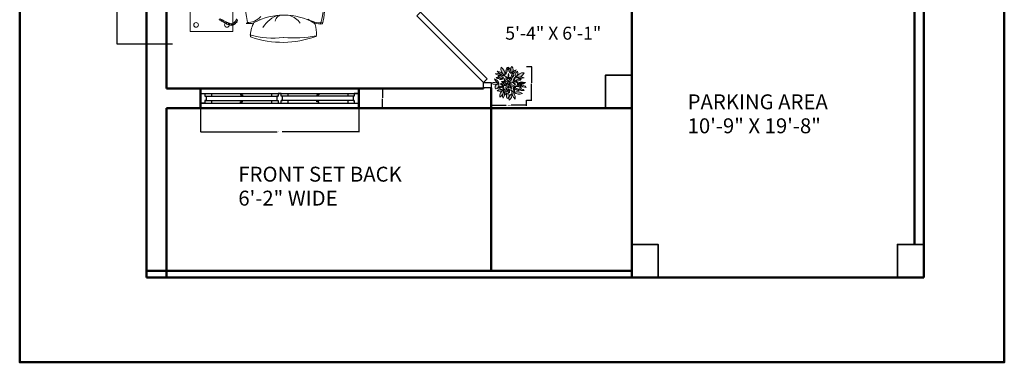
# Model space of a CAD drawing. Units: inches. Extents: x 64 to 1167, y 117 to 939.
# Tile 1 of 56: x 64 to 513, y 117 to 272. Entities that reach past the tile are written whole.
import ezdxf

# ---------------------------------------------------------------- set-up
doc = ezdxf.new("R2010")
doc.units = ezdxf.units.IN
doc.header["$MEASUREMENT"] = 0
for name, color, linetype, lineweight in [('A-ANNO-DIMS', 2, 'Continuous', 18), ('A-ANNO-TEXT', 7, 'Continuous', 25), ('A-ANNO-TTLB', 7, 'Continuous', 50), ('A-COLS', 7, 'Continuous', 35), ('A-DOOR', 4, 'Continuous', 25), ('A-FURN', 8, 'Continuous', 18), ('A-GLAZ', 4, 'Continuous', 25), ('A-WALL', 7, 'Continuous', 50)]:
    doc.layers.add(name, color=color, linetype=linetype, lineweight=lineweight)
doc.styles.get("Standard").update_dxf_attribs({"font": 'arial.ttf'})
doc.dimstyles.get("Standard").update_dxf_attribs({"dimtxt": 0.18, "dimasz": 0.18, "dimexe": 0.18, "dimexo": 0.0625, "dimgap": 0.09, "dimtad": 0, "dimtih": 1, "dimtoh": 1, "dimdec": 4, "dimzin": 0, "dimdsep": 46, "dimtxsty": 'Standard', "dimcen": 0.09, "dimadec": 0, "dimazin": 0, "dimtfac": 1, "dimtdec": 4, "dimtofl": 0, "dimtmove": 0, "dimatfit": 3, "dimfxl": 1, "dimtolj": 1, "dimtzin": 0, "dimarcsym": 0})

# ---------------------------------------------------------------- blocks, each defined once
blk = doc.blocks.new('A$C68901CC0')
for p, q in [((10.95, 26.62), (12.35, 28.01)), ((36.01, 1.56), (10.95, 26.62)), ((12.35, 28.01), (37.4, 2.95)), ((0, 2.95), (0, 0)), ((1.97, 2.95), (0, 2.95)), ((0, 0), (1.97, 0)), ((1.97, 0), (1.97, 2.95)), ((37.4, 2.95), (36.01, 1.56)), ((37.4, 2.95), (37.4, 0)), ((39.37, 2.95), (37.4, 2.95)), ((37.4, 0), (39.37, 0)), ((39.37, 0), (39.37, 2.95))]:
    blk.add_line(p, q)
blk.add_arc((37.4, 2.95), 35.43, 135, 180)
blk = doc.blocks.new("W-6'")
for p, q in [((0, 9), (0, 0)), ((0, 9), (72, 9)), ((72, 9), (72, 0)), ((0, 6.75), (72, 6.75)), ((2, 5.5), (35.25, 5.5)), ((70, 5.5), (36.75, 5.5)), ((0, 2.25), (72, 2.25)), ((0, 0), (72, 0)), ((2, 3.5), (35.25, 3.5)), ((70, 3.5), (36.75, 3.5))]:
    blk.add_line(p, q)
for points in [[(0, 2.25), (0, 6.75), (2, 6.75), (2, 5.5), (2.5, 5.5), (2.5, 3.5), (2, 3.5), (2, 2.25), (0, 2.25)], [(5, 6.75), (5, 5.5)], [(18.125, 6.75), (18.125, 6.125), (19.125, 6.125), (19.125, 5.5)], [(32.25, 6.75), (32.25, 5.5)], [(39.75, 6.75), (39.75, 5.5)], [(53.875, 6.75), (53.875, 6.125), (52.875, 6.125), (52.875, 5.5)], [(67, 6.75), (67, 5.5)], [(72, 2.25), (72, 6.75), (70, 6.75), (70, 5.5), (69.5, 5.5), (69.5, 3.5), (70, 3.5), (70, 2.25), (72, 2.25)], [(5, 3.5), (5, 2.25)], [(18.125, 2.25), (18.125, 2.875), (19.125, 2.875), (19.125, 3.5)], [(32.25, 3.5), (32.25, 2.25)], [(39.75, 3.5), (39.75, 2.25)], [(53.875, 2.25), (53.875, 2.875), (52.875, 2.875), (52.875, 3.5)], [(67, 3.5), (67, 2.25)]]:
    blk.add_lwpolyline(points)
blk.add_lwpolyline([(36.75, 6.75), (35.25, 6.75), (35.25, 5.5), (34.75, 5.5), (34.75, 3.5), (35.25, 3.5), (35.25, 2.25), (36.75, 2.25), (36.75, 3.5), (37.25, 3.5), (37.25, 5.5), (36.75, 5.5)], close=True)
blk = doc.blocks.new('A$C28C76B35')
for p, q in [((66.74, 162.49, -24.36), (86.28, 162.49, -24.36)), ((66.74, 137.72, -24.36), (66.74, 162.49, -24.36)), ((86.28, 162.49, -24.36), (86.28, 137.72, -24.36)), ((64.63, 157.46, -55.71), (64.77, 157.76, -55.71)), ((65, 157.04, -55.71), (64.63, 157.46, -55.71)), ((64.77, 157.76, -55.71), (65.33, 157.7, -55.71)), ((64.85, 158.09, -55.71), (65.11, 158.39, -55.71)), ((65.33, 157.7, -55.71), (64.85, 158.09, -55.71)), ((65.11, 158.39, -55.71), (65.61, 158.17, -55.71)), ((65.63, 157.82, -55.71), (65.16, 156.74, -55.71)), ((65.39, 158.69, -55.71), (65.61, 158.93, -55.71)), ((65.61, 158.17, -55.71), (65.39, 158.69, -55.71)), ((65.61, 158.93, -55.71), (66.11, 158.67, -55.71)), ((66.43, 158.63, -55.71), (65.63, 157.82, -55.71)), ((65.94, 159.21, -55.71), (66.32, 159.36, -55.71)), ((66.11, 158.67, -55.71), (65.94, 159.21, -55.71)), ((66.32, 159.36, -55.71), (66.82, 158.91, -55.71)), ((67.82, 158.89, -55.71), (66.43, 158.63, -55.71)), ((66.79, 159.49, 50.88), (67.17, 159.56, 50.88)), ((66.82, 158.91, -55.71), (66.8, 159.49, -55.71)), ((67.17, 159.56, -55.71), (67.45, 159.08, -55.71)), ((67.45, 159.08, -55.71), (67.62, 159.65, -55.71)), ((67.61, 159.66, 50.88), (68.08, 159.57, 50.88)), ((69.56, 158.28, -55.71), (67.82, 158.89, -55.71)), ((68.08, 159.56, -55.71), (68.08, 159.06, -55.71)), ((68.08, 159.06, -55.71), (68.45, 159.45, -55.71)), ((68.44, 159.45, 50.88), (68.87, 159.32, 50.88)), ((68.88, 159.32, -55.71), (68.86, 158.73, -55.71)), ((68.86, 158.73, -55.71), (69.06, 159.26, -55.71)), ((69.06, 159.26, -55.71), (69.62, 159.1, -55.71)), ((69.62, 159.1, -55.71), (69.56, 158.54, -55.71)), ((69.56, 158.54, -55.71), (70.1, 158.87, -55.71)), ((70.64, 157.69, -55.71), (69.56, 158.28, -55.71)), ((70.1, 158.87, -55.71), (70.4, 158.67, -55.71)), ((70.4, 158.67, -55.71), (70.25, 158.15, -55.71)), ((70.25, 158.15, -55.71), (70.75, 158.43, -55.71)), ((70.79, 157.74, -55.71), (70.64, 157.69, -55.71)), ((70.75, 158.43, -55.71), (71.14, 158.22, -55.71)), ((70.83, 157.61, -55.71), (70.79, 157.74, -55.71)), ((71.59, 157.22, -55.71), (70.83, 157.61, -55.71)), ((71.14, 158.22, -55.71), (70.98, 157.72, -55.71)), ((70.98, 157.72, -55.71), (71.4, 158.06, -55.71)), ((71.4, 158.06, -55.71), (71.81, 157.87, -55.71)), ((71.81, 157.87, -55.71), (71.59, 157.37, -55.71)), ((71.59, 157.37, -55.71), (72.01, 157.76, -55.71)), ((72.59, 156.63, -55.71), (71.59, 157.22, -55.71)), ((72.01, 157.76, -55.71), (72.31, 157.61, -55.71)), ((72.31, 157.61, -55.71), (72.14, 157.07, -55.71)), ((72.14, 157.07, -55.71), (72.68, 157.37, -55.71)), ((72.68, 157.37, -55.71), (72.96, 157.22, -55.71)), ((72.96, 157.22, -55.71), (72.81, 156.74, -55.71))]:
    blk.add_line(p, q)
for centre in [(69.47, 159.47, -27.2), (83.55, 159.47, -27.2)]:
    blk.add_circle(centre, 1.07)
for centre, radius, start, end in [((44.19, 123.6, -100.22), 43.8, 71.1157, 110.2204), ((29.35, 164.01, -100.22), 0.74, 113.3322, 161.3637), ((45.92, 164.21, -100.22), 17.27, 179.879, 196.6328), ((29.34, 164.01, -100.22), 0.74, 114.0758, 156.3315), ((38.67, 116, -100.22), 49.39, 84.253, 101.4358), ((48.54, 128.59, -100.22), 36.87, 73.3816, 97.55), ((47.45, 164.2, -100.22), 11.31, 332.1884, 2.3768), ((58.09, 164.35, -100.22), 0.74, 25.7033, 68.2144), ((90.3, 145.69, -100.22), 65.74, 168.3019, 188.2166), ((77.92, 144.85, -100.22), 52.97, 164.4911, 189.2138), ((26.82, 151.23, -100.22), 7.84, 69.9615, 96.5551), ((26.79, 147.45, -100.22), 11.05, 58.4292, 93.73), ((30.11, 159.24, -100.22), 0.74, 177.437, 237.6208), ((30.11, 159.24, -100.22), 0.74, 178.0201, 240.7828), ((30.13, 158.98, -100.22), 0.74, 184.7243, 243.4779), ((43.65, 183.47, -100.22), 28.49, 240.7828, 298.0488), ((27.78, 151.92, -100.22), 6.89, 46.9453, 51.4779), ((44.46, 165.16, -100.22), 10.65, 217.955, 250.4125), ((44.45, 157.99, -100.22), 3.03, 261.0221, 354.0715), ((42.56, 166.77, -100.22), 12.19, 284.9836, 329.7062), ((60.3, 149.77, -100.22), 8.6, 88.8733, 136.7696), ((59.08, 151.92, -100.22), 6.89, 128.5221, 133.0547), ((56.72, 158.98, -100.22), 0.74, 296.5221, 355.2757), ((59.4, 151.99, -100.22), 6.91, 78.8784, 107.2062), ((-1.21, 144.26, -100.22), 62.88, 353.0352, 12.9689)]:
    blk.add_arc(centre, radius, start, end)
blk = doc.blocks.new('A$C172C5132')
at = {"linetype": 'ByBlock'}
h = blk.add_hatch(color=256, dxfattribs=at)
h.set_gradient(color1=(12, 110, 14), color2=(39, 78, 9), tint=1, name='HEMISPHERICAL')
h.paths.add_polyline_path([(0.0278, 0.1013, 0.287265), (0.0517, 0.0926, 0.287265)])
h.paths.add_polyline_path([(0.0334, 0.0874, 0.245454), (0.05, 0.09, 0.245454)])
h.paths.add_polyline_path([(0.053, 0.0887, 0.362884), (0.0729, 0.0765, -0.000877), (0.073, 0.0766, 0.362272)])
h.paths.add_polyline_path([(0.053, 0.0808, 0.33327), (0.0599, 0.073, 0.33327)])
h.paths.add_polyline_path([(0.043, 0.0778, 0.302945), (0.0552, 0.0735, 0.302945)])
h.paths.add_polyline_path([(0.0378, 0.0674, 0.378763), (0.0534, 0.0687, 0.378763)])
h.paths.add_polyline_path([(0.0317, 0.0482, 0.247698), (0.0464, 0.0594, -0.032946), (0.0468, 0.0616, 0.274039)])
h.paths.add_polyline_path([(0.0169, 0.0474, 0.549808), (0.0308, 0.0669, 0.549808)])
h.paths.add_polyline_path([(0, 0.0704, 0.297781), (0.0304, 0.069, 0.297781)])
h.paths.add_polyline_path([(0.013, 0.0887, 0.248111), (0.0313, 0.0713, 0.248111)])
h.paths.add_polyline_path([(0.0204, 0.0943, 0.290415), (0.033, 0.0908, 0.290415)])
h.paths.add_polyline_path([(0.0165, 0.1104, 0.175406), (0.0437, 0.1045, -0.037323), (0.0372, 0.1086, 0.129374)])
h.paths.add_polyline_path([(0.0252, 0.1213, 0.085647), (0.0372, 0.1086, -0.054384), (0.0452, 0.1048), (0.0452, 0.1048, -0.009351), (0.0437, 0.1045, 0.060507), (0.0552, 0.1), (0.0556, 0.1006, 0.185254)])
h.paths.add_polyline_path([(0.0408, 0.1378, 0.313266), (0.0566, 0.1033), (0.0567, 0.1033, 0.313266)])
h.paths.add_polyline_path([(0.0712, 0.0891), (0.0716, 0.0886, 0.230232), (0.0821, 0.0965, 0.230232)])
h.paths.add_polyline_path([(0.0877, 0.0943), (0.0881, 0.0941, 0.179345), (0.0947, 0.1078, 0.179345)])
h.paths.add_polyline_path([(0.1008, 0.0968), (0.1016, 0.0965, 0.378282), (0.1103, 0.1204, 0.378282)])
h = blk.add_hatch(color=256, dxfattribs=at)
h.set_gradient(color1=(15, 138, 17), color2=(46, 92, 10), tint=1, name='HEMISPHERICAL')
h.paths.add_polyline_path([(0.0849, 0.0409, 0.236282), (0.1, 0.0045, 0.236282)])
h.paths.add_polyline_path([(0.0951, 0.0322, 0.290628), (0.1303, 0.0274, 0.290628)])
h.paths.add_polyline_path([(0.0751, 0, 0.364082), (0.0843, 0.0256, 0.364082)])
h.paths.add_polyline_path([(0.0708, 0.0309, 0.428936), (0.0669, 0.0061, 0.428936)])
h.paths.add_polyline_path([(0.0526, 0.0469, 0.243055), (0.0634, 0.0209, 0.243055)])
h.paths.add_polyline_path([(0.0509, 0.0311, -0.075692), (0.0478, 0.0235, 0.164666), (0.0495, 0.0087, 0.298636), (0.053, 0.0339, 0.03785)])
h.paths.add_polyline_path([(0.0356, 0.0126, 0.152567), (0.0478, 0.0235, -0.089408), (0.0509, 0.0311, 0.1023), (0.0513, 0.0422, 0.341288)])
h.paths.add_polyline_path([(0.0248, 0.0387, 0.299202), (0.0498, 0.0428, 0.299202)])
h.paths.add_polyline_path([(0.0475, 0.0637, 0.031182), (0.0468, 0.0616, -0.006707), (0.0473, 0.0617), (0.0473, 0.0617), (0.0473, 0.0617, -0.03138), (0.0464, 0.0594, 0.214704), (0.0508, 0.0461, 0.282795)])
h.paths.add_polyline_path([(0.0643, 0.0658, 0.211659), (0.0625, 0.043, 0.281051), (0.0686, 0.0717, 0.038772), (0.0659, 0.0683, -0.044717)])
h.paths.add_polyline_path([(0.053, 0.0591, 0.203733), (0.0643, 0.0658, -0.026656), (0.0659, 0.0683, 0.062829), (0.0673, 0.0723, 0.318582)])
h.paths.add_polyline_path([(0.0695, 0.0439, 0.403257), (0.076, 0.0304, 0.403257)])
h.paths.add_polyline_path([(0.0652, 0.0343, 0.302607), (0.0678, 0.0439, 0.302607)])
h.paths.add_polyline_path([(0.0708, 0.0452, 0.20419), (0.0817, 0.0413, 0.20419)])
h.paths.add_polyline_path([(0.0817, 0.0582, 0.262138), (0.0834, 0.0452, 0.262138)])
h.paths.add_polyline_path([(0.0721, 0.05, 0.44636), (0.0791, 0.0622, 0.44636)])
h.paths.add_polyline_path([(0.0934, 0.0526, 0.247085), (0.1173, 0.0391, 0.247085)])
h.paths.add_polyline_path([(0.0712, 0.0682, 0.171467), (0.1021, 0.0548, 0.171467)])
h.paths.add_polyline_path([(0.0747, 0.07, 0.259278), (0.0934, 0.0765, 0.259278)])
h.paths.add_polyline_path([(0.0917, 0.073, 0.365639), (0.1012, 0.0652, 0.365639)])
h.paths.add_polyline_path([(0.0934, 0.0795, 0.243415), (0.1108, 0.0735, 0.243415)])
h.paths.add_polyline_path([(0.1012, 0.0591, 0.307451), (0.1129, 0.0574, 0.307451)])
h.paths.add_polyline_path([(0.1086, 0.0674, 0.209633), (0.1264, 0.0496, 0.209633)])
h.paths.add_polyline_path([(0.1208, 0.0652, 0.21311), (0.1464, 0.0526, 0.21311)])
h.paths.add_polyline_path([(0.116, 0.0469, 0.265719), (0.1373, 0.04, 0.265719)])
h.paths.add_polyline_path([(0.1012, 0.0804, 0.271534), (0.1255, 0.0874, 0.271534)])
h.paths.add_polyline_path([(0.1204, 0.0965, -0.10541), (0.1084, 0.0945, 0.018052), (0.1055, 0.0935, 0.194763), (0.1373, 0.0935, 0.102488)])
h.paths.add_polyline_path([(0.1055, 0.0948, 0.024701), (0.1084, 0.0945, -0.072299), (0.1204, 0.0965, 0.220444), (0.1373, 0.1143, 0.361284)])
h.paths.add_polyline_path([(0.0921, 0.0808, 0.244188), (0.0999, 0.0961, 0.244188)])
h.paths.add_polyline_path([(0.0873, 0.1078, 0.236039), (0.1042, 0.1265, 0.236039)])
h.paths.add_polyline_path([(0.0843, 0.1056, 0.271887), (0.0875, 0.0951, 0.271887)])
h.paths.add_polyline_path([(0.073, 0.0766, -0.001193), (0.073, 0.0765, 0.325344), (0.0864, 0.0931, 0.324468)])
h.paths.add_polyline_path([(0.0713, 0.0905, 0.143951), (0.0721, 0.1108, 0.143951)])
h.paths.add_polyline_path([(0.0591, 0.1, 0.207976), (0.0691, 0.0891, 0.207976)])
h.paths.add_polyline_path([(0.0604, 0.1065, 0.190107), (0.0669, 0.1374, 0.190107)])
h.paths.add_polyline_path([(0.0708, 0.1374, 0.252904), (0.0838, 0.1095, 0.067921), (0.0831, 0.1182, -0.074796), (0.0813, 0.124, 0.134159)])
h.paths.add_polyline_path([(0.0813, 0.124, -0.046564), (0.0831, 0.1182, 0.072445), (0.0864, 0.1134, 0.391074), (0.0864, 0.1408, 0.229731)])
h = blk.add_hatch(color=256)
h.set_gradient(color1=(12, 110, 14), color2=(39, 78, 9), tint=1, name='HEMISPHERICAL')
h.paths.add_polyline_path([(0.0925, 0.0526), (0.092, 0.0525, 0.192472), (0.0973, 0.0343, 0.192472)])
h = blk.add_hatch(color=256, dxfattribs=at)
h.set_gradient(color1=(12, 110, 14), color2=(39, 78, 9), tint=1, name='HEMISPHERICAL')
h.paths.add_polyline_path([(0.1077, 0.0699), (0.1077, 0.0695, 0.262244), (0.1429, 0.073, 0.262244)])
for p, q in [((0.0552, 0.1), (0.0556, 0.1006)), ((0.0566, 0.1033), (0.0567, 0.1033)), ((0.0716, 0.0886), (0.0712, 0.0891)), ((0.0881, 0.0941), (0.0877, 0.0943)), ((0.1016, 0.0965), (0.1008, 0.0968)), ((0.0925, 0.0526), (0.092, 0.0525)), ((0.1077, 0.0695), (0.1077, 0.0699))]:
    blk.add_line(p, q, dxfattribs=at)
for centre, radius, start, end in [((0.0736, 0.1319), 0.0333, 169.7437, 239.3198), ((0.024, 0.1091), 0.0333, 349.9797, 59.5558), ((0.1028, 0.1137), 0.043, 146.5506, 189.6063), ((0.0245, 0.1302), 0.043, 326.5506, 9.6063), ((0.1031, 0.1355), 0.0323, 176.7146, 233.4855), ((0.0516, 0.1114), 0.0323, 356.7146, 53.4855), ((0.1013, 0.1271), 0.0202, 137.2816, 222.7184), ((0.0716, 0.1271), 0.0202, 317.2816, 42.7184), ((0.1145, 0.1002), 0.0282, 111.2499, 164.3738), ((0.0771, 0.1341), 0.0282, 291.2499, 344.3738), ((0.0386, 0.0972), 0.027, 198.5093, 254.2466), ((0.0057, 0.0627), 0.027, 18.5093, 74.2466), ((0.0235, 0.0702), 0.0408, 57.8807, 99.8189), ((0.0382, 0.145), 0.0408, 237.8807, 279.8189), ((0.024, 0.0827), 0.0122, 42.1798, 106.9561), ((0.0295, 0.1025), 0.0122, 222.1798, 286.9561), ((0.0135, 0.0713), 0.0513, 34.8518, 76.8329), ((0.0679, 0.1498), 0.0513, 213.7346, 255.7157), ((0.0328, 0.0779), 0.024, 37.9495, 102.0596), ((0.0467, 0.116), 0.024, 217.9495, 282.0596), ((0.0442, 0.0729), 0.018, 71.397, 126.5601), ((0.0392, 0.1045), 0.018, 251.397, 306.5601), ((0.0557, 0.0706), 0.0182, 18.7265, 98.5819), ((0.0703, 0.0945), 0.0182, 198.7265, 278.5819), ((0.0516, 0.083), 0.0185, 19.0975, 66.0922), ((0.0766, 0.106), 0.0185, 199.0975, 246.0922), ((0.1064, 0.0993), 0.0362, 161.3279, 196.3785), ((0.037, 0.102), 0.0362, 339.0434, 14.094), ((0.0682, 0.094), 0.0182, 278.3256, 1.7816), ((0.0843, 0.0816), 0.015, 98.3028, 150.1644), ((0.0688, 0.1034), 0.015, 280.7404, 332.602), ((0.0911, 0.0756), 0.0182, 100.5964, 184.0524), ((0.0949, 0.1031), 0.0109, 166.6712, 231.5788), ((0.0769, 0.0976), 0.0109, 342.6051, 47.5126), ((0.1094, 0.0917), 0.0218, 132.3809, 173.0513), ((0.073, 0.1098), 0.0218, 313.9894, 354.6599), ((0.0813, 0.096), 0.0186, 305.3547, 0.2444), ((0.1106, 0.0809), 0.0186, 125.3547, 180.2444), ((0.1189, 0.1032), 0.0192, 116.5049, 199.3878), ((0.1193, 0.0631), 0.025, 75.5726, 136.3385), ((0.1074, 0.1046), 0.025, 255.5726, 316.3385), ((0.0924, 0.1134), 0.0192, 298.5878, 21.4707), ((0.1332, 0.0855), 0.0291, 81.9405, 161.3964), ((0.1096, 0.1236), 0.0291, 261.9405, 341.3964), ((0.1214, 0.0543), 0.0422, 67.9577, 112.0423), ((0.1214, 0.1326), 0.0422, 247.9577, 292.0423), ((0.0141, 0.0464), 0.0278, 52.0955, 120.5238), ((0.0163, 0.093), 0.0278, 234.1936, 302.622), ((0.0301, 0.0527), 0.0142, 86.9965, 202.2058), ((0.0177, 0.0616), 0.0142, 266.9965, 22.2058), ((0.0404, 0.0217), 0.0231, 65.4893, 132.7752), ((0.0341, 0.0598), 0.0231, 246.1459, 313.4318), ((0.0285, 0.0678), 0.0198, 279.3324, 342.1699), ((0.0506, 0.0422), 0.0198, 99.3324, 162.1699), ((0.0626, 0.0173), 0.0273, 114.4303, 189.807), ((0.0243, 0.0375), 0.0273, 294.4303, 9.807), ((0.0463, 0.0592), 0.0118, 53.2772, 136.2565), ((0.0449, 0.0769), 0.0118, 233.2772, 316.2565), ((0.0458, 0.0665), 0.0116, 36.6262, 104.0418), ((0.0523, 0.0847), 0.0116, 216.6262, 284.0418), ((0.0634, 0.0576), 0.0171, 157.7122, 222.4235), ((0.0348, 0.0521), 0.0171, 339.261, 43.9723), ((0.0832, 0.0444), 0.0308, 175.2839, 229.9285), ((0.0327, 0.0234), 0.0308, 355.2839, 49.9285), ((0.0512, 0.0723), 0.00872, 4.751, 78.4779), ((0.0617, 0.0816), 0.00872, 184.751, 258.4779), ((0.0508, 0.0758), 0.0168, 277.3883, 349.0703), ((0.0694, 0.0556), 0.0168, 96.3902, 168.0722), ((0.0891, 0.0524), 0.0281, 136.6356, 199.4278), ((0.0421, 0.0624), 0.0281, 316.6356, 19.4278), ((0.0736, 0.0372), 0.00894, 131.0823, 198.427), ((0.0593, 0.0411), 0.00894, 311.0823, 18.427), ((0.0798, 0.0405), 0.0108, 161.8817, 249.7301), ((0.0658, 0.0338), 0.0108, 341.8817, 69.7301), ((0.0808, 0.056), 0.0147, 227.1077, 273.2701), ((0.0716, 0.0305), 0.0147, 47.1077, 93.2701), ((0.1057, 0.1051), 0.0505, 226.9394, 265.8583), ((0.0676, 0.0179), 0.0505, 46.9394, 85.8583), ((0.081, 0.053), 0.00941, 102.1635, 198.3798), ((0.0701, 0.0592), 0.00941, 282.1635, 18.3798), ((0.0899, 0.0564), 0.0204, 80.1717, 138.3136), ((0.0782, 0.09), 0.0204, 260.1717, 318.3136), ((0.0941, 0.0533), 0.0134, 158.2119, 216.9673), ((0.056, 0.0075), 0.0441, 356.0096, 54.5768), ((0.0709, 0.0502), 0.0134, 338.2119, 36.9673), ((0.0918, 0.0634), 0.00957, 10.523, 90.8605), ((0.1011, 0.0748), 0.00957, 190.523, 270.8605), ((0.1173, 0.05), 0.0254, 174.4977, 218.0761), ((0.0721, 0.0375), 0.0254, 352.8778, 36.4562), ((0.0962, 0.0597), 0.02, 43.3367, 98.0592), ((0.108, 0.0933), 0.02, 223.3367, 278.0592), ((0.1181, 0.0686), 0.0294, 212.8184, 268.3343), ((0.0925, 0.0232), 0.0294, 32.8184, 88.3343), ((0.1058, 0.0496), 0.0106, 47.3873, 115.7476), ((0.1084, 0.0669), 0.0106, 227.3873, 295.7476), ((0.1281, 0.0402), 0.036, 65.6693, 124.4476), ((0.1222, 0.1025), 0.036, 246.2552, 305.0335), ((0.0972, 0.0382), 0.0314, 21.3015, 68.66), ((0.1378, 0.0788), 0.0314, 201.3015, 248.66), ((0.1205, 0.0249), 0.0226, 42.1437, 101.6667), ((0.1327, 0.0621), 0.0226, 222.1437, 281.6667), ((0.1195, 0.0302), 0.035, 39.7488, 87.8702), ((0.1477, 0.0876), 0.035, 219.7488, 267.8702), ((0.0705, 0.0186), 0.0232, 138.8969, 205.4069), ((0.032, 0.0239), 0.0232, 318.8969, 25.4069), ((0.0806, 0.0166), 0.0173, 124.6008, 217.4658), ((0.0571, 0.0203), 0.0173, 304.6008, 37.4658), ((0.095, 0.0074), 0.0212, 120.4086, 200.4312), ((0.0644, 0.0183), 0.0212, 300.4086, 20.4312), ((0.1289, 0.0379), 0.0441, 176.0096, 229.186), ((0.109, 0.0021), 0.0331, 49.8506, 114.6719), ((0.1165, 0.0575), 0.0331, 229.8506, 294.6719)]:
    blk.add_arc(centre, radius, start, end, dxfattribs=at)
blk = doc.blocks.new('*D64')
at = {"layer": 'A-ANNO-DIMS', "color": 0, "lineweight": -2, "transparency": 16777216}
for p, q in [((279.11, 235.82), (279.11, 233.32)), ((279.29, 233.5), (285.93, 233.5)), ((294.85, 233.5), (288.21, 233.5)), ((295.03, 235.82), (295.03, 233.32))]:
    blk.add_line(p, q, dxfattribs=at)
for points in [[(279.29, 233.53), (279.29, 233.47), (279.11, 233.5)], [(294.85, 233.53), (294.85, 233.47), (295.03, 233.5)]]:
    blk.add_solid(points, dxfattribs=at)
at = {"layer": 'Defpoints', "color": 0, "lineweight": -2, "transparency": 16777216}
for p in [(279.11, 235.88), (295.03, 235.88), (295.03, 233.5)]:
    blk.add_point(p, dxfattribs=at)
at = {"layer": 'A-ANNO-DIMS', "color": 0, "transparency": 16777216, "insert": (287.07, 233.5), "char_height": 0.18, "attachment_point": 5}
blk.add_mtext('\\A1;PLANTER 16 TYP.', dxfattribs=at)
blk = doc.blocks.new('*D65')
at = {"layer": 'A-ANNO-DIMS', "color": 0, "lineweight": -2, "transparency": 16777216}
for p, q in [((295.1, 251.21), (297.6, 251.21)), ((297.42, 251.03), (297.42, 243.73)), ((297.42, 236.06), (297.42, 243.36)), ((295.1, 235.88), (297.6, 235.88))]:
    blk.add_line(p, q, dxfattribs=at)
for points in [[(297.39, 251.03), (297.45, 251.03), (297.42, 251.21)], [(297.39, 236.06), (297.45, 236.06), (297.42, 235.88)]]:
    blk.add_solid(points, dxfattribs=at)
at = {"layer": 'Defpoints', "color": 0, "lineweight": -2, "transparency": 16777216}
for p in [(295.03, 251.21), (297.42, 251.21), (295.03, 235.88)]:
    blk.add_point(p, dxfattribs=at)
at = {"layer": 'A-ANNO-DIMS', "color": 0, "transparency": 16777216, "insert": (297.42, 243.54), "char_height": 0.18, "attachment_point": 5}
blk.add_mtext('\\A1;15 TYP.', dxfattribs=at)
blk = doc.blocks.new('*D72')
at = {"layer": 'A-ANNO-DIMS', "color": 0, "lineweight": -2, "transparency": 16777216}
for p, q in [((146.71, 232.14), (146.71, 221.22)), ((218.71, 232.14), (218.71, 221.22)), ((146.89, 221.4), (181.61, 221.4)), ((218.53, 221.4), (183.81, 221.4))]:
    blk.add_line(p, q, dxfattribs=at)
for points in [[(146.89, 221.43), (146.89, 221.37), (146.71, 221.4)], [(218.53, 221.43), (218.53, 221.37), (218.71, 221.4)]]:
    blk.add_solid(points, dxfattribs=at)
at = {"layer": 'Defpoints', "color": 0, "lineweight": -2, "transparency": 16777216}
for p in [(146.71, 232.2), (218.71, 232.2), (218.71, 221.4)]:
    blk.add_point(p, dxfattribs=at)
at = {"layer": 'A-ANNO-DIMS', "color": 0, "transparency": 16777216, "insert": (182.71, 221.4), "char_height": 0.18, "attachment_point": 5}
blk.add_mtext("\\A1;WINDOW W-6' 72", dxfattribs=at)
blk = doc.blocks.new('*D73')
at = {"layer": 'A-ANNO-DIMS', "color": 0, "lineweight": -2, "transparency": 16777216}
for p, q in [((218.77, 241.2), (229.69, 241.2)), ((229.51, 241.02), (229.51, 236.88)), ((229.51, 232.38), (229.51, 236.52)), ((218.77, 232.2), (229.69, 232.2))]:
    blk.add_line(p, q, dxfattribs=at)
for points in [[(229.48, 241.02), (229.54, 241.02), (229.51, 241.2)], [(229.48, 232.38), (229.54, 232.38), (229.51, 232.2)]]:
    blk.add_solid(points, dxfattribs=at)
at = {"layer": 'Defpoints', "color": 0, "lineweight": -2, "transparency": 16777216}
for p in [(218.71, 241.2), (229.51, 241.2), (218.71, 232.2)]:
    blk.add_point(p, dxfattribs=at)
at = {"layer": 'A-ANNO-DIMS', "color": 0, "transparency": 16777216, "insert": (229.51, 236.7), "char_height": 0.18, "attachment_point": 5}
blk.add_mtext('\\A1;9', dxfattribs=at)
blk = doc.blocks.new('*D82')
at = {"layer": 'A-ANNO-DIMS', "color": 0, "lineweight": -2, "transparency": 16777216}
for p, q in [((133.91, 429.56), (108.54, 429.56)), ((108.72, 429.38), (108.72, 345.6)), ((108.72, 261.45), (108.72, 345.23)), ((133.91, 261.27), (108.54, 261.27))]:
    blk.add_line(p, q, dxfattribs=at)
for points in [[(108.69, 429.38), (108.75, 429.38), (108.72, 429.56)], [(108.69, 261.45), (108.75, 261.45), (108.72, 261.27)]]:
    blk.add_solid(points, dxfattribs=at)
at = {"layer": 'Defpoints', "color": 0, "lineweight": -2, "transparency": 16777216}
for p in [(133.97, 429.56), (108.72, 261.27), (133.97, 261.27)]:
    blk.add_point(p, dxfattribs=at)
at = {"layer": 'A-ANNO-DIMS', "color": 0, "transparency": 16777216, "insert": (108.72, 345.42), "char_height": 0.18, "attachment_point": 5}
blk.add_mtext('\\A1;SOFA SET 168', dxfattribs=at)

msp = doc.modelspace()

# ---------------------------------------------------------------- linework, layer by layer
at = {"layer": 'A-ANNO-TTLB'}
msp.add_lwpolyline([(64.31, 939.22), (512.77, 939.22), (512.77, 116.55), (64.31, 116.55)], close=True, dxfattribs=at)
at = {"layer": 'A-COLS'}
for points in [[(343.11, 232.2), (331.11, 232.2), (331.11, 247.2), (343.11, 247.2)], [(355.11, 155.2), (343.11, 155.2), (343.11, 170.2), (355.11, 170.2)], [(476.11, 155.2), (464.11, 155.2), (464.11, 170.2), (476.11, 170.2)]]:
    msp.add_lwpolyline(points, close=True, dxfattribs=at)
at = {"layer": 'A-WALL'}
for p, q in [((122.11, 863.2), (122.11, 155.2)), ((476.11, 863.2), (476.11, 155.2)), ((131.11, 433.2), (131.11, 241.2)), ((343.11, 314.2), (343.11, 155.2)), ((471.79, 314.2), (471.79, 170.2)), ((275.11, 241.2), (131.11, 241.2)), ((146.71, 241.2), (146.71, 232.2)), ((218.71, 241.2), (218.71, 232.2)), ((275.52, 241.2), (275.11, 241.2)), ((275.52, 241.43), (275.52, 241.2)), ((279.11, 241.43), (279.11, 158.2)), ((131.11, 232.2), (131.11, 155.2)), ((343.11, 232.2), (131.11, 232.2)), ((343.11, 158.2), (122.11, 158.2)), ((476.11, 155.2), (122.11, 155.2))]:
    msp.add_line(p, q, dxfattribs=at)

# ---------------------------------------------------------------- block references
at = {"layer": 'A-DOOR', "xscale": -1.213305874571074, "yscale": 1.213305874571074, "zscale": 1.213305874571074, "rotation": 90}
msp.add_blockref('A$C68901CC0', (279.11, 289.2), dxfattribs=at)
at = {"layer": 'A-FURN', "rotation": 180}
msp.add_blockref('A$C28C76B35', (228.19, 429.56, 28.15), dxfattribs=at)
at = {"layer": 'A-FURN', "xscale": 108.7946212322529, "yscale": 108.7946212322529, "zscale": 108.7946212322529}
msp.add_blockref('A$C172C5132', (279.11, 235.88), dxfattribs=at)
at = {"layer": 'A-GLAZ'}
msp.add_blockref("W-6'", (146.71, 232.2), dxfattribs=at)

# ---------------------------------------------------------------- texts
at = {"layer": 'A-ANNO-TEXT'}
for s, height, p in [(' 5\'-4" X 6\'-1"', 5.8926, (283.67, 263.38)), ('PARKING AREA', 6.7927, (368.53, 231.7)), ('10\'-9" X 19\'-8"', 6.7927, (368.53, 220.79)), ('FRONT SET BACK', 6.7927, (163.89, 198.77)), ('6\'-2" WIDE', 6.793, (163.89, 187.86))]:
    msp.add_text(s, height=height, dxfattribs=at).set_placement(p)

# ---------------------------------------------------------------- dimensions: what is measured, and where the dimension line sits
at = {"layer": 'A-ANNO-DIMS'}
for base, p1, p2, angle, text, picture, middle in [((108.72, 261.27), (133.97, 429.56), (133.97, 261.27), 270, 'SOFA SET <>', '*D82', (108.72, 345.42)), ((297.42, 251.21), (295.03, 235.88), (295.03, 251.21), 90, '<> TYP.', '*D65', (297.42, 243.54))]:
    dim = msp.add_linear_dim(base=base, p1=p1, p2=p2, angle=angle, text=text, dimstyle='Standard', override={"dimdec": 0, "dimlfac": 1, "dimrnd": 0, "dimzin": 0, "dimdsep": 46, "dimlunit": 2}, dxfattribs=at)
    dim.commit()
    dim.dimension.update_dxf_attribs({"geometry": picture, "text_midpoint": middle})
dim = msp.add_linear_dim(base=(229.51, 241.2), p1=(218.71, 232.2), p2=(218.71, 241.2), angle=90, dimstyle='Standard', override={"dimdec": 0, "dimlfac": 1, "dimrnd": 0, "dimzin": 0, "dimdsep": 46, "dimlunit": 2}, dxfattribs=at)
dim.commit()
dim.dimension.update_dxf_attribs({"geometry": '*D73', "text_midpoint": (229.51, 236.7)})
for base, p1, p2, text, picture, middle in [((295.03, 233.5), (279.11, 235.88), (295.03, 235.88), 'PLANTER <> TYP.', '*D64', (287.07, 233.5)), ((218.71, 221.4), (146.71, 232.2), (218.71, 232.2), "WINDOW W-6' <>", '*D72', (182.71, 221.4))]:
    dim = msp.add_linear_dim(base=base, p1=p1, p2=p2, text=text, dimstyle='Standard', override={"dimdec": 0, "dimlfac": 1, "dimrnd": 0, "dimzin": 0, "dimdsep": 46, "dimlunit": 2}, dxfattribs=at)
    dim.commit()
    dim.dimension.update_dxf_attribs({"geometry": picture, "text_midpoint": middle})

doc.saveas('drawing.dxf')
